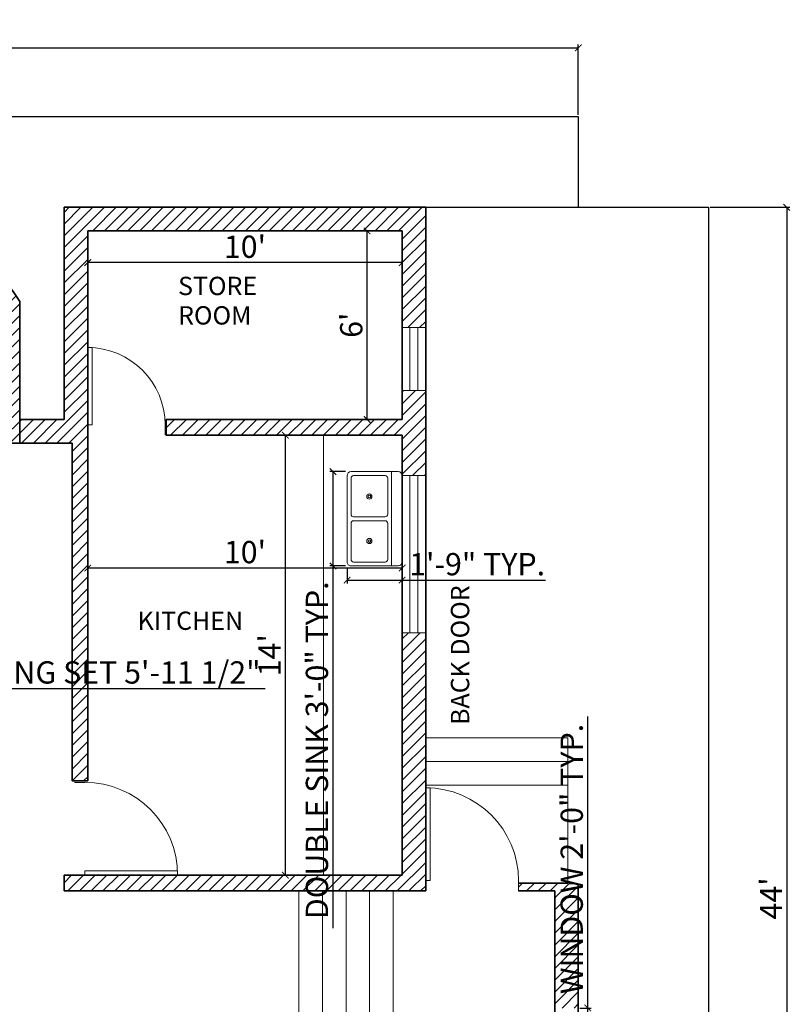
# Model space of a CAD drawing. Units: inches. Extents: x 3799 to 20199, y 1682 to 8087.
# Tile 20 of 30: x 14582 to 14876, y 2852 to 3227. Entities that reach past the tile are written whole.
import ezdxf

# ---------------------------------------------------------------- set-up
doc = ezdxf.new("R2010")
doc.units = ezdxf.units.IN
for name, color, linetype, lineweight in [('A-ANNO-DIMS', 2, 'Continuous', 18), ('A-AREA-IDEN', 7, 'Continuous', 18), ('A-DOOR', 3, 'Continuous', 18), ('A-FLOR-CASE', 32, 'Continuous', 18), ('A-FLOR-FIXT', 9, 'Continuous', 18), ('A-FLOR-STRS', 41, 'Continuous', 18), ('A-GLAZ', 152, 'Continuous', 18), ('A-WALL', 7, 'Continuous', 35), ('A-WALL-PATT', 252, 'Continuous', 13), ('C-PROP', 7, 'Continuous', 25)]:
    doc.layers.add(name, color=color, linetype=linetype, lineweight=lineweight)
doc.styles.get("Standard").update_dxf_attribs({"font": 'arial.ttf'})
doc.dimstyles.new('ISO-25', dxfattribs={"dimtxt": 8.5, "dimasz": 2.5, "dimexe": 1.25, "dimexo": 0.625, "dimtad": 1, "dimdec": 0, "dimlunit": 3, "dimtxsty": 'Standard', "dimblk": 'ARCHTICK', "dimcen": 2.5, "dimadec": 0, "dimazin": 0, "dimtfac": 1, "dimtdec": 0, "dimtmove": 0, "dimatfit": 3, "dimfxl": 1, "dimarcsym": 0})

# ---------------------------------------------------------------- blocks, each defined once
blk = doc.blocks.new('*U97')
for p, q in [((0, 0), (0, -100)), ((900, 0), (900, -100))]:
    blk.add_line(p, q)
blk.add_lwpolyline([(0, 0), (0, 900), (43.75, 900), (43.75, 0)], close=True)
blk.add_arc((0, 0), 900, 0, 90)
blk = doc.blocks.new('*U7')
for p, q in [((0, 0), (0, -100)), ((750, 0), (750, -100))]:
    blk.add_line(p, q)
blk.add_lwpolyline([(0, 0), (0, 750), (43.75, 750), (43.75, 0)], close=True)
blk.add_arc((0, 0), 750, 0, 90)
blk = doc.blocks.new('*U94')
for p, q in [((0, 0), (0, 100)), ((900, 0), (900, 100))]:
    blk.add_line(p, q)
blk.add_lwpolyline([(0, 0), (0, -900), (43.75, -900), (43.75, 0)], close=True)
blk.add_arc((0, 0), 900, 270, 0)
blk = doc.blocks.new('Sink-double - 36 in top')
for p, q in [((-18, -4), (18, -4)), ((-0.75, -18.5), (-0.75, -6.5)), ((0.75, -6.5), (0.75, -18.5))]:
    blk.add_line(p, q)
for points in [[(-16.5, 0), (16.5, 0)], [(-18, -19.5), (-18, -1.5)], [(18, -1.5), (18, -19.5)], [(-16.5, -18.5), (-16.5, -6.5)], [(-15.5, -5.5), (-1.75, -5.5)], [(1.75, -5.5), (15.5, -5.5)], [(16.5, -6.5), (16.5, -18.5)], [(16.5, -21), (-16.5, -21)], [(-1.75, -19.5), (-15.5, -19.5)], [(15.5, -19.5), (1.75, -19.5)]]:
    blk.add_lwpolyline(points)
for centre, radius in [((-8.5, -12.5), 1), ((-8.5, -12.5), 0.5), ((8.5, -12.5), 1), ((8.5, -12.5), 0.5)]:
    blk.add_circle(centre, radius)
for centre, radius, start, end in [((-16.5, -1.5), 1.5, 90, 180), ((16.5, -1.5), 1.5, 0, 90), ((-15.5, -6.5), 1, 90, 180), ((-1.75, -6.5), 1, 0, 90), ((1.75, -6.5), 1, 90, 180), ((15.5, -6.5), 1, 0, 90), ((-15.5, -18.5), 1, 180, 270), ((-1.75, -18.5), 1, 270, 0), ((1.75, -18.5), 1, 180, 270), ((15.5, -18.5), 1, 270, 0), ((-16.5, -19.5), 1.5, 180, 270), ((16.5, -19.5), 1.5, 270, 0)]:
    blk.add_arc(centre, radius, start, end)
blk = doc.blocks.new('_ArchTick')
at = {"color": 0, "linetype": 'ByBlock', "const_width": 0.15}
blk.add_lwpolyline([(-0.5, -0.5), (0.5, 0.5)], dxfattribs=at)
blk = doc.blocks.new('*D117')
at = {"layer": 'A-ANNO-DIMS', "color": 0, "lineweight": -2, "transparency": 16777216}
for p, q in [((14608.2, 3146.16), (14608.2, 3133.44)), ((14728.2, 3146.16), (14728.2, 3133.44)), ((14728.2, 3134.69), (14608.2, 3134.69))]:
    blk.add_line(p, q, dxfattribs=at)
at = {"layer": 'Defpoints', "color": 0, "transparency": 16777216}
for p in [(14608.2, 3146.79), (14728.2, 3146.79), (14608.2, 3134.69)]:
    blk.add_point(p, dxfattribs=at)
at = {"layer": 'A-ANNO-DIMS', "color": 0, "lineweight": -2, "transparency": 16777216, "xscale": 2.5, "yscale": 2.5, "zscale": 2.5, "rotation": 180}
blk.add_blockref('_ArchTick', (14608.2, 3134.69), dxfattribs=at)
at = {"layer": 'A-ANNO-DIMS', "color": 0, "lineweight": -2, "transparency": 16777216, "xscale": 2.5, "yscale": 2.5, "zscale": 2.5}
blk.add_blockref('_ArchTick', (14728.2, 3134.69), dxfattribs=at)
at = {"layer": 'A-ANNO-DIMS', "color": 0, "transparency": 16777216, "insert": (14668.2, 3139.65), "char_height": 8.5, "attachment_point": 5}
blk.add_mtext("10'", dxfattribs=at)
blk = doc.blocks.new('*D118')
at = {"layer": 'A-ANNO-DIMS', "color": 0, "lineweight": -2, "transparency": 16777216}
for p, q in [((14727.58, 3146.79), (14713.6, 3146.79)), ((14714.85, 3074.79), (14714.85, 3146.79)), ((14727.58, 3074.79), (14713.6, 3074.79))]:
    blk.add_line(p, q, dxfattribs=at)
at = {"layer": 'Defpoints', "color": 0, "transparency": 16777216}
for p in [(14714.85, 3146.79), (14728.2, 3146.79), (14728.2, 3074.79)]:
    blk.add_point(p, dxfattribs=at)
at = {"layer": 'A-ANNO-DIMS', "color": 0, "lineweight": -2, "transparency": 16777216, "xscale": 2.5, "yscale": 2.5, "zscale": 2.5}
for p, rotation in [((14714.85, 3146.79), 90), ((14714.85, 3074.79), 270)]:
    blk.add_blockref('_ArchTick', p, dxfattribs=dict(at, rotation=rotation))
at = {"layer": 'A-ANNO-DIMS', "color": 0, "transparency": 16777216, "insert": (14709.88, 3110.79), "char_height": 8.5, "attachment_point": 5, "rotation": 90}
blk.add_mtext("6'", dxfattribs=at)
blk = doc.blocks.new('*D119')
at = {"layer": 'A-ANNO-DIMS', "color": 0, "lineweight": -2, "transparency": 16777216}
for p, q in [((14608.2, 2937.41), (14608.2, 3019.34)), ((14728.2, 2937.41), (14728.2, 3019.34)), ((14608.2, 3018.09), (14728.2, 3018.09))]:
    blk.add_line(p, q, dxfattribs=at)
at = {"layer": 'Defpoints', "color": 0, "transparency": 16777216}
for p in [(14728.2, 3018.09), (14608.2, 2936.79), (14728.2, 2936.79)]:
    blk.add_point(p, dxfattribs=at)
at = {"layer": 'A-ANNO-DIMS', "color": 0, "lineweight": -2, "transparency": 16777216, "xscale": 2.5, "yscale": 2.5, "zscale": 2.5, "rotation": 180}
blk.add_blockref('_ArchTick', (14608.2, 3018.09), dxfattribs=at)
at = {"layer": 'A-ANNO-DIMS', "color": 0, "lineweight": -2, "transparency": 16777216, "xscale": 2.5, "yscale": 2.5, "zscale": 2.5}
blk.add_blockref('_ArchTick', (14728.2, 3018.09), dxfattribs=at)
at = {"layer": 'A-ANNO-DIMS', "color": 0, "transparency": 16777216, "insert": (14668.2, 3023.06), "char_height": 8.5, "attachment_point": 5}
blk.add_mtext("10'", dxfattribs=at)
blk = doc.blocks.new('*D120')
at = {"layer": 'A-ANNO-DIMS', "color": 0, "lineweight": -2, "transparency": 16777216}
for p, q in [((14697.58, 3068.79), (14682.36, 3068.79)), ((14683.61, 3068.79), (14683.61, 2900.79)), ((14697.58, 2900.79), (14682.36, 2900.79))]:
    blk.add_line(p, q, dxfattribs=at)
at = {"layer": 'Defpoints', "color": 0, "transparency": 16777216}
for p in [(14698.2, 3068.79), (14683.61, 2900.79), (14698.2, 2900.79)]:
    blk.add_point(p, dxfattribs=at)
at = {"layer": 'A-ANNO-DIMS', "color": 0, "lineweight": -2, "transparency": 16777216, "xscale": 2.5, "yscale": 2.5, "zscale": 2.5}
for p, rotation in [((14683.61, 3068.79), 90), ((14683.61, 2900.79), 270)]:
    blk.add_blockref('_ArchTick', p, dxfattribs=dict(at, rotation=rotation))
at = {"layer": 'A-ANNO-DIMS', "color": 0, "transparency": 16777216, "insert": (14678.72, 2984.79), "char_height": 8.5, "attachment_point": 5, "rotation": 90}
blk.add_mtext("14'", dxfattribs=at)
blk = doc.blocks.new('*D121')
at = {"layer": 'A-ANNO-DIMS', "color": 0, "lineweight": -2, "transparency": 16777216}
for p, q in [((14845.83, 3155.79), (14876.24, 3155.79)), ((14874.99, 3155.79), (14874.99, 2628.09)), ((14845.83, 2628.09), (14876.24, 2628.09))]:
    blk.add_line(p, q, dxfattribs=at)
at = {"layer": 'Defpoints', "color": 0, "transparency": 16777216}
for p in [(14845.2, 3155.79), (14845.2, 2628.09), (14874.99, 2628.09)]:
    blk.add_point(p, dxfattribs=at)
at = {"layer": 'A-ANNO-DIMS', "color": 0, "lineweight": -2, "transparency": 16777216, "xscale": 2.5, "yscale": 2.5, "zscale": 2.5}
for p, rotation in [((14874.99, 3155.79), 90), ((14874.99, 2628.09), 270)]:
    blk.add_blockref('_ArchTick', p, dxfattribs=dict(at, rotation=rotation))
at = {"layer": 'A-ANNO-DIMS', "color": 0, "transparency": 16777216, "insert": (14870.11, 2891.94), "char_height": 8.5, "attachment_point": 5, "rotation": 90}
blk.add_mtext("44'", dxfattribs=at)
blk = doc.blocks.new('*D122')
at = {"layer": 'A-ANNO-DIMS', "color": 0, "lineweight": -2, "transparency": 16777216}
for p, q in [((14309.46, 3191.05), (14309.46, 3217.92)), ((14795.46, 3191.05), (14795.46, 3217.92)), ((14309.46, 3216.67), (14795.46, 3216.67))]:
    blk.add_line(p, q, dxfattribs=at)
at = {"layer": 'Defpoints', "color": 0, "transparency": 16777216}
for p in [(14795.46, 3216.67), (14309.46, 3190.42), (14795.46, 3190.42)]:
    blk.add_point(p, dxfattribs=at)
at = {"layer": 'A-ANNO-DIMS', "color": 0, "lineweight": -2, "transparency": 16777216, "xscale": 2.5, "yscale": 2.5, "zscale": 2.5, "rotation": 180}
blk.add_blockref('_ArchTick', (14309.46, 3216.67), dxfattribs=at)
at = {"layer": 'A-ANNO-DIMS', "color": 0, "lineweight": -2, "transparency": 16777216, "xscale": 2.5, "yscale": 2.5, "zscale": 2.5}
blk.add_blockref('_ArchTick', (14795.46, 3216.67), dxfattribs=at)
at = {"layer": 'A-ANNO-DIMS', "color": 0, "transparency": 16777216, "insert": (14552.46, 3221.64), "char_height": 8.5, "attachment_point": 5}
blk.add_mtext('40\'-6"', dxfattribs=at)
blk = doc.blocks.new('WIN-24IN-9IN-FRAME')
for p, q in [((0, 24), (9, 24)), ((3, 0), (3, 24)), ((6, 0), (6, 24)), ((0, 0), (9, 0))]:
    blk.add_line(p, q)
blk = doc.blocks.new('WIN-60IN-9IN-FRAME')
for p, q in [((0, 9), (0, 0)), ((60, 9), (60, 0)), ((60, 6), (0, 6)), ((60, 3), (0, 3))]:
    blk.add_line(p, q)
blk = doc.blocks.new('*D242')
at = {"layer": 'A-ANNO-DIMS', "color": 0, "lineweight": -2, "transparency": 16777216}
for p, q in [((14799.06, 2850.1), (14799.06, 2961.41)), ((14796.09, 2850.1), (14800.31, 2850.1)), ((14799.06, 2826.1), (14799.06, 2850.1)), ((14796.09, 2826.1), (14800.31, 2826.1))]:
    blk.add_line(p, q, dxfattribs=at)
at = {"layer": 'Defpoints', "color": 0, "transparency": 16777216}
for p in [(14795.46, 2850.1), (14799.06, 2850.1), (14795.46, 2826.1)]:
    blk.add_point(p, dxfattribs=at)
at = {"layer": 'A-ANNO-DIMS', "color": 0, "lineweight": -2, "transparency": 16777216, "xscale": 2.5, "yscale": 2.5, "zscale": 2.5}
for p, rotation in [((14799.06, 2850.1), 90), ((14799.06, 2826.1), 270)]:
    blk.add_blockref('_ArchTick', p, dxfattribs=dict(at, rotation=rotation))
at = {"layer": 'A-ANNO-DIMS', "color": 0, "transparency": 16777216, "insert": (14794.04, 2907), "char_height": 8.5, "attachment_point": 5, "rotation": 90}
blk.add_mtext('WINDOW 2\'-0" TYP.', dxfattribs=at)
blk = doc.blocks.new('*D292')
at = {"layer": 'A-ANNO-DIMS', "color": 0, "lineweight": -2, "transparency": 16777216}
for p, q in [((14480.74, 2982.21), (14480.74, 2970.84)), ((14552.38, 2982.21), (14552.38, 2970.84)), ((14480.74, 2972.09), (14552.38, 2972.09)), ((14552.38, 2972.09), (14675.97, 2972.09))]:
    blk.add_line(p, q, dxfattribs=at)
at = {"layer": 'Defpoints', "color": 0, "transparency": 16777216}
for p in [(14480.74, 2982.83), (14552.38, 2982.83), (14552.38, 2972.09)]:
    blk.add_point(p, dxfattribs=at)
at = {"layer": 'A-ANNO-DIMS', "color": 0, "lineweight": -2, "transparency": 16777216, "xscale": 2.5, "yscale": 2.5, "zscale": 2.5, "rotation": 180}
blk.add_blockref('_ArchTick', (14480.74, 2972.09), dxfattribs=at)
at = {"layer": 'A-ANNO-DIMS', "color": 0, "lineweight": -2, "transparency": 16777216, "xscale": 2.5, "yscale": 2.5, "zscale": 2.5}
blk.add_blockref('_ArchTick', (14552.38, 2972.09), dxfattribs=at)
at = {"layer": 'A-ANNO-DIMS', "color": 0, "transparency": 16777216, "insert": (14615.42, 2977.11), "char_height": 8.5, "attachment_point": 5}
blk.add_mtext('DINING SET 5\'-11 1/2"', dxfattribs=at)
blk = doc.blocks.new('*D298')
at = {"layer": 'A-ANNO-DIMS', "color": 0, "lineweight": -2, "transparency": 16777216}
for p, q in [((14706.58, 3054.88), (14700.55, 3054.88)), ((14701.8, 3054.88), (14701.8, 3018.88)), ((14706.58, 3018.88), (14700.55, 3018.88)), ((14701.8, 3018.88), (14701.8, 2880.6))]:
    blk.add_line(p, q, dxfattribs=at)
at = {"layer": 'Defpoints', "color": 0, "transparency": 16777216}
for p in [(14707.2, 3054.88), (14701.8, 3018.88), (14707.2, 3018.88)]:
    blk.add_point(p, dxfattribs=at)
at = {"layer": 'A-ANNO-DIMS', "color": 0, "lineweight": -2, "transparency": 16777216, "xscale": 2.5, "yscale": 2.5, "zscale": 2.5}
for p, rotation in [((14701.8, 3054.88), 90), ((14701.8, 3018.88), 270)]:
    blk.add_blockref('_ArchTick', p, dxfattribs=dict(at, rotation=rotation))
at = {"layer": 'A-ANNO-DIMS', "color": 0, "transparency": 16777216, "insert": (14696.78, 2948.49), "char_height": 8.5, "attachment_point": 5, "rotation": 90}
blk.add_mtext('DOUBLE SINK 3\'-0" TYP.', dxfattribs=at)
blk = doc.blocks.new('*D299')
at = {"layer": 'A-ANNO-DIMS', "color": 0, "lineweight": -2, "transparency": 16777216}
for p, q in [((14707.2, 3018.26), (14707.2, 3012.23)), ((14728.2, 3018.26), (14728.2, 3012.23)), ((14707.2, 3013.48), (14728.2, 3013.48)), ((14728.2, 3013.48), (14782.96, 3013.48))]:
    blk.add_line(p, q, dxfattribs=at)
at = {"layer": 'Defpoints', "color": 0, "transparency": 16777216}
for p in [(14707.2, 3018.88), (14728.2, 3018.88), (14728.2, 3013.48)]:
    blk.add_point(p, dxfattribs=at)
at = {"layer": 'A-ANNO-DIMS', "color": 0, "lineweight": -2, "transparency": 16777216, "xscale": 2.5, "yscale": 2.5, "zscale": 2.5, "rotation": 180}
blk.add_blockref('_ArchTick', (14707.2, 3013.48), dxfattribs=at)
at = {"layer": 'A-ANNO-DIMS', "color": 0, "lineweight": -2, "transparency": 16777216, "xscale": 2.5, "yscale": 2.5, "zscale": 2.5}
blk.add_blockref('_ArchTick', (14728.2, 3013.48), dxfattribs=at)
at = {"layer": 'A-ANNO-DIMS', "color": 0, "transparency": 16777216, "insert": (14756.83, 3018.45), "char_height": 8.5, "attachment_point": 5}
blk.add_mtext('1\'-9" TYP.', dxfattribs=at)

msp = doc.modelspace()

# ---------------------------------------------------------------- hatches: boundary and pattern name
at = {"layer": 'A-WALL-PATT'}
h = msp.add_hatch(dxfattribs=at)
h.set_pattern_fill('ANSI31', color=256)
h.paths.add_polyline_path([(14318.46, 2965.3), (14318.46, 2981.76), (14420.46, 2981.76), (14420.46, 2987.76), (14318.46, 2987.76), (14318.46, 3083.76), (14369.36, 3083.76), (14369.36, 3092.76), (14309.46, 3092.76), (14309.46, 2953.3), (14318.46, 2953.3)])
h.paths.add_polyline_path([(14456.46, 3092.76), (14393.36, 3092.76), (14393.36, 3083.76), (14450.46, 3083.76), (14450.46, 2987.76), (14450.46, 2981.76), (14450.46, 2889.09), (14456.46, 2889.09), (14456.46, 2891.79), (14539.2, 2891.79), (14539.2, 2945.79), (14533.2, 2945.79), (14533.2, 2897.79), (14456.46, 2897.79), (14456.46, 3065.79), (14474.23, 3065.79), (14474.23, 3074.79), (14456.46, 3074.79)])
h.paths.add_polyline_path([(14480.23, 3119.94, -0.534305), (14576.23, 3119.94), (14576.23, 3065.79), (14582.23, 3065.79), (14582.23, 3119.79, 0.570302), (14474.23, 3119.79), (14474.23, 3065.79), (14480.23, 3065.79)])
h.paths.add_polyline_path([(14608.2, 3146.79), (14728.2, 3146.79), (14728.2, 3109.9), (14737.2, 3109.9), (14737.2, 3155.79), (14599.2, 3155.79), (14599.2, 3074.79), (14582.23, 3074.79), (14582.23, 3065.79), (14602.2, 3065.79), (14602.2, 2936.79), (14608.2, 2936.79)])
h.paths.add_polyline_path([(14737.2, 3085.9), (14728.2, 3085.9), (14728.2, 3074.79), (14638.2, 3074.79), (14638.2, 3068.79), (14728.2, 3068.79), (14728.2, 3053.38), (14737.2, 3053.38)], flags=17)
h.paths.add_polyline_path([(14737.2, 2993.38), (14728.2, 2993.38), (14728.2, 2900.79), (14599.2, 2900.79), (14599.2, 2894.79), (14737.2, 2894.79)])
h.paths.add_polyline_path([(14795.46, 2897.45), (14791.43, 2897.45), (14791.43, 2897.79), (14772.64, 2897.79), (14772.64, 2894.79), (14786.46, 2894.79), (14786.46, 2850.1), (14795.46, 2850.1)])
h.paths.add_polyline_path([(14795.46, 2826.1), (14786.46, 2826.1), (14786.46, 2787.09), (14645.38, 2787.09), (14645.38, 2781.09), (14648.46, 2781.09), (14648.46, 2740.52), (14654.46, 2740.52), (14654.46, 2781.09), (14795.46, 2781.09)])
h.paths.add_polyline_path([(14654.46, 2680.52), (14648.46, 2680.52), (14648.46, 2637.09), (14599.58, 2637.09), (14599.58, 2628.09), (14654.46, 2628.09)])
h.paths.add_polyline_path([(14539.58, 2637.09), (14504.46, 2637.09), (14504.46, 2781.09), (14609.38, 2781.09), (14609.38, 2787.09), (14498.46, 2787.09), (14498.46, 2637.09), (14456.79, 2637.09), (14456.79, 2628.09), (14539.58, 2628.09)])
h.paths.add_polyline_path([(14396.79, 2637.09), (14384.79, 2637.09), (14354.46, 2637.09), (14354.46, 2739.09), (14456.46, 2739.09), (14456.46, 2745.09), (14354.46, 2745.09), (14354.46, 2785.72), (14345.46, 2785.72), (14345.46, 2628.09), (14396.79, 2628.09)])
h.paths.add_polyline_path([(14456.46, 2853.09), (14450.46, 2853.09), (14318.46, 2853.09), (14318.46, 2893.3), (14309.46, 2893.3), (14309.46, 2847.09), (14345.46, 2847.09), (14345.46, 2809.72), (14354.46, 2809.72), (14354.46, 2847.09), (14450.46, 2847.09), (14450.46, 2775.09), (14456.46, 2775.09)])

# ---------------------------------------------------------------- linework, layer by layer
at = {"layer": 'A-FLOR-CASE'}
msp.add_line((14698.2, 2900.79), (14698.2, 3068.79), dxfattribs=at)
at = {"layer": 'A-FLOR-STRS'}
for p, q in [((14791.43, 2953.2), (14737.2, 2953.2)), ((14791.43, 2897.45), (14791.43, 2953.2)), ((14791.43, 2944.2), (14737.2, 2944.2)), ((14791.43, 2935.2), (14737.2, 2935.2)), ((14688.78, 2894.79), (14688.78, 2842.79)), ((14697.78, 2894.79), (14697.78, 2842.79)), ((14706.78, 2894.79), (14706.78, 2842.79)), ((14715.78, 2894.79), (14715.78, 2842.79)), ((14724.78, 2894.79), (14724.78, 2787.09)), ((14791.43, 2897.45), (14795.46, 2897.45))]:
    msp.add_line(p, q, dxfattribs=at)
at = {"layer": 'A-WALL'}
for p, q in [((14737.2, 3155.79), (14599.2, 3155.79)), ((14599.2, 3074.79), (14599.2, 3155.79)), ((14737.2, 2894.79), (14737.2, 3155.79)), ((14728.2, 3146.79), (14608.2, 3146.79)), ((14608.2, 2936.79), (14608.2, 3146.79)), ((14728.2, 3074.79), (14728.2, 3146.79)), ((14582.23, 3065.79), (14582.23, 3119.79)), ((14599.2, 3074.79), (14582.23, 3074.79)), ((14728.2, 3074.79), (14638.2, 3074.79)), ((14638.2, 3068.79), (14638.2, 3074.79)), ((14728.2, 3068.79), (14638.2, 3068.79)), ((14728.2, 2900.79), (14728.2, 3068.79)), ((14602.2, 3065.79), (14474.23, 3065.79)), ((14602.2, 2936.79), (14602.2, 3065.79)), ((14608.2, 2936.79), (14602.2, 2936.79)), ((14599.2, 2894.79), (14599.2, 2900.79)), ((14728.2, 2900.79), (14599.2, 2900.79)), ((14737.2, 2894.79), (14599.2, 2894.79)), ((14772.64, 2897.79), (14791.43, 2897.79)), ((14772.64, 2894.79), (14786.46, 2894.79)), ((14786.46, 2787.09), (14786.46, 2894.79)), ((14795.46, 2781.09), (14795.46, 2897.45))]:
    msp.add_line(p, q, dxfattribs=at)
msp.add_arc((14528.23, 3087.84), 62.74, 30.6076, 149.3924, dxfattribs=at)
at = {"layer": 'C-PROP'}
for p, q in [((14309.46, 3190.42), (14795.46, 3190.42)), ((14795.46, 3190.42), (14795.46, 3155.79)), ((14737.2, 3155.79), (14845.2, 3155.79)), ((14845.2, 3155.79), (14845.2, 2628.09))]:
    msp.add_line(p, q, dxfattribs=at)

# ---------------------------------------------------------------- block references
at = {"layer": 'A-DOOR', "xscale": 0.0393700787401575, "yscale": 0.0393700787401575, "zscale": 0.0393700787401575}
for name, p in [('*U7', (14608.2, 3072.73)), ('*U97', (14737.2, 2898.73))]:
    msp.add_blockref(name, p, dxfattribs=at)
at = {"layer": 'A-DOOR', "xscale": 0.0393700787401575, "yscale": 0.0393700787401575, "zscale": 0.0393700787401575, "rotation": 90}
msp.add_blockref('*U94', (14607.08, 2900.79), dxfattribs=at)
at = {"layer": 'A-FLOR-FIXT', "rotation": 270}
msp.add_blockref('Sink-double - 36 in top', (14728.2, 3036.88), dxfattribs=at)
at = {"layer": 'A-GLAZ'}
msp.add_blockref('WIN-24IN-9IN-FRAME', (14728.2, 3085.9), dxfattribs=at)
at = {"layer": 'A-GLAZ', "rotation": 90}
msp.add_blockref('WIN-60IN-9IN-FRAME', (14737.2, 2993.38), dxfattribs=at)

# ---------------------------------------------------------------- texts
at = {"layer": 'A-AREA-IDEN'}
for s, rotation, p in [('STORE', 0.0019, (14642.68, 3122.28)), ('ROOM', 0.0019, (14642.68, 3111.04)), ('BACK DOOR', 90.0019, (14753.82, 2958.16)), ('KITCHEN', 0.0019, (14627.23, 2994.46))]:
    msp.add_text(s, height=7, rotation=rotation, dxfattribs=at).set_placement(p)

# ---------------------------------------------------------------- dimensions: what is measured, and where the dimension line sits
at = {"layer": 'A-ANNO-DIMS'}
for base, p1, p2, picture, middle in [((14795.46, 3216.67), (14309.46, 3190.42), (14795.46, 3190.42), '*D122', (14552.46, 3221.64)), ((14608.2, 3134.69), (14728.2, 3146.79), (14608.2, 3146.79), '*D117', (14668.2, 3139.65)), ((14728.2, 3018.09), (14608.2, 2936.79), (14728.2, 2936.79), '*D119', (14668.2, 3023.06))]:
    dim = msp.add_linear_dim(base=base, p1=p1, p2=p2, dimstyle='ISO-25', override={"dimclrd": 0, "dimclre": 0, "dimclrt": 0}, dxfattribs=at)
    dim.commit()
    dim.dimension.update_dxf_attribs({"geometry": picture, "text_midpoint": middle})
for base, p1, p2, picture, middle in [((14874.99, 2628.09), (14845.2, 3155.79), (14845.2, 2628.09), '*D121', (14870.11, 2891.94)), ((14714.85, 3146.79), (14728.2, 3074.79), (14728.2, 3146.79), '*D118', (14709.88, 3110.79)), ((14683.61, 2900.79), (14698.2, 3068.79), (14698.2, 2900.79), '*D120', (14678.72, 2984.79))]:
    dim = msp.add_linear_dim(base=base, p1=p1, p2=p2, angle=90, dimstyle='ISO-25', override={"dimclrd": 0, "dimclre": 0, "dimclrt": 0}, dxfattribs=at)
    dim.commit()
    dim.dimension.update_dxf_attribs({"geometry": picture, "text_midpoint": middle})
for base, p1, p2, angle, text, picture, middle in [((14701.8, 3018.88), (14707.2, 3054.88), (14707.2, 3018.88), 270, 'DOUBLE SINK <> TYP.', '*D298', (14696.78, 2948.49)), ((14799.06, 2850.1), (14795.46, 2826.1), (14795.46, 2850.1), 90, 'WINDOW <> TYP.', '*D242', (14794.04, 2907))]:
    dim = msp.add_linear_dim(base=base, p1=p1, p2=p2, angle=angle, text=text, dimstyle='ISO-25', override={"dimdec": 1, "dimlfac": 1, "dimrnd": 0, "dimzin": 1, "dimdsep": 46, "dimlunit": 4, "dimfrac": 2}, dxfattribs=at)
    dim.commit()
    dim.dimension.update_dxf_attribs({"geometry": picture, "text_midpoint": middle})
for base, p1, p2, text, picture, middle in [((14728.2, 3013.48), (14707.2, 3018.88), (14728.2, 3018.88), '<> TYP.', '*D299', (14756.83, 3018.45)), ((14552.38, 2972.09), (14480.74, 2982.83), (14552.38, 2982.83), 'DINING SET <>', '*D292', (14615.42, 2977.11))]:
    dim = msp.add_linear_dim(base=base, p1=p1, p2=p2, text=text, dimstyle='ISO-25', override={"dimdec": 1, "dimlfac": 1, "dimrnd": 0, "dimzin": 1, "dimdsep": 46, "dimlunit": 4, "dimfrac": 2}, dxfattribs=at)
    dim.commit()
    dim.dimension.update_dxf_attribs({"geometry": picture, "text_midpoint": middle})

doc.saveas('drawing.dxf')
